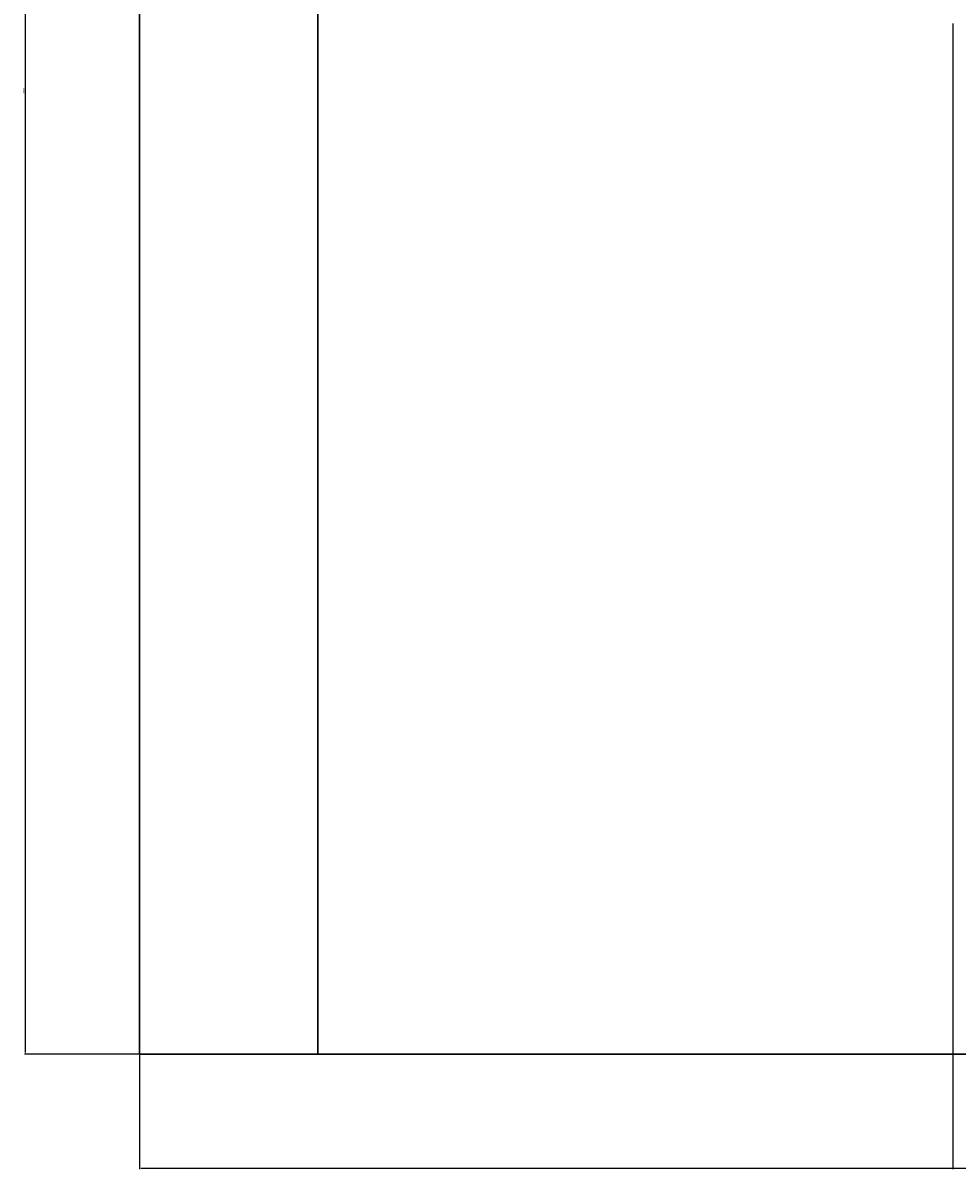
# Model space of a CAD drawing. Units: millimetres. Extents: x 2332 to 5836, y -853 to 2199.
# Tile 1 of 16: x 2332 to 3641, y -853 to 753. Entities that reach past the tile are written whole.
import ezdxf

# ---------------------------------------------------------------- set-up
doc = ezdxf.new("R2010")
doc.units = ezdxf.units.MM
doc.layers.add('A-ANNO-DIMS', color=2, linetype='Continuous', lineweight=18)
doc.layers.add('A-WALL', color=8, linetype='Continuous', lineweight=30)
doc.styles.get("Standard").update_dxf_attribs({"font": 'arial.ttf'})
doc.dimstyles.new('ISO-25', dxfattribs={"dimtxt": 2.5, "dimasz": 2.5, "dimexe": 1.25, "dimexo": 0.625, "dimtad": 1, "dimtxsty": 'Standard', "dimcen": 2.5, "dimadec": 0, "dimazin": 0, "dimtfac": 1, "dimtmove": 0, "dimatfit": 3, "dimfxl": 1, "dimarcsym": 0})

# ---------------------------------------------------------------- blocks, each defined once
blk = doc.blocks.new('*D15')
at = {"layer": 'A-ANNO-DIMS', "color": 0, "lineweight": -2, "transparency": 16777216}
for p, q in [((2495, -692.8), (2495, -853.1)), ((5675, -692.8), (5675, -853.1)), ((2497.5, -851.8), (5672.5, -851.8))]:
    blk.add_line(p, q, dxfattribs=at)
at = {"layer": 'A-ANNO-DIMS', "color": 0, "transparency": 16777216}
for points in [[(2497.5, -851.4), (2497.5, -852.3), (2495, -851.8)], [(5672.5, -851.4), (5672.5, -852.3), (5675, -851.8)]]:
    blk.add_solid(points, dxfattribs=at)
at = {"layer": 'Defpoints', "color": 0, "transparency": 16777216}
for p in [(2495, -692.2), (5675, -692.2), (5675, -851.8)]:
    blk.add_point(p, dxfattribs=at)
at = {"layer": 'A-ANNO-DIMS', "color": 0, "transparency": 16777216, "insert": (4085, -849.9), "char_height": 2.5, "attachment_point": 5}
blk.add_mtext('3180', dxfattribs=at)
blk = doc.blocks.new('*D16')
at = {"layer": 'A-ANNO-DIMS', "color": 0, "lineweight": -2, "transparency": 16777216}
for p, q in [((2494.4, 2007.8), (2334.1, 2007.8)), ((2335.4, -689.7), (2335.4, 2005.3)), ((2494.4, -692.2), (2334.1, -692.2))]:
    blk.add_line(p, q, dxfattribs=at)
at = {"layer": 'A-ANNO-DIMS', "color": 0, "transparency": 16777216}
for points in [[(2335, 2005.3), (2335.8, 2005.3), (2335.4, 2007.8)], [(2335, -689.7), (2335.8, -689.7), (2335.4, -692.2)]]:
    blk.add_solid(points, dxfattribs=at)
at = {"layer": 'Defpoints', "color": 0, "transparency": 16777216}
for p in [(2335.4, 2007.8), (2495, 2007.8), (2495, -692.2)]:
    blk.add_point(p, dxfattribs=at)
at = {"layer": 'A-ANNO-DIMS', "color": 0, "transparency": 16777216, "insert": (2333.5, 657.8), "char_height": 2.5, "attachment_point": 5, "rotation": 90}
blk.add_mtext('2700', dxfattribs=at)
blk = doc.blocks.new('*D22')
at = {"layer": 'A-ANNO-DIMS', "color": 0, "lineweight": -2, "transparency": 16777216}
for p, q in [((3635, 752.2), (3635, -853.1)), ((4785, 752.2), (4785, -853.1)), ((3637.5, -851.8), (4782.5, -851.8))]:
    blk.add_line(p, q, dxfattribs=at)
at = {"layer": 'A-ANNO-DIMS', "color": 0, "transparency": 16777216}
for points in [[(3637.5, -851.4), (3637.5, -852.3), (3635, -851.8)], [(4782.5, -851.4), (4782.5, -852.3), (4785, -851.8)]]:
    blk.add_solid(points, dxfattribs=at)
at = {"layer": 'Defpoints', "color": 0, "transparency": 16777216}
for p in [(3635, 752.8), (4785, 752.8), (4785, -851.8)]:
    blk.add_point(p, dxfattribs=at)
at = {"layer": 'A-ANNO-DIMS', "color": 0, "transparency": 16777216, "insert": (4210, -849.9), "char_height": 2.5, "attachment_point": 5}
blk.add_mtext('1150', dxfattribs=at)

msp = doc.modelspace()

# ---------------------------------------------------------------- linework, layer by layer
at = {"layer": 'A-WALL'}
for p, q in [((2495.04, -692.197), (2495.04, 2007.803)), ((2745.04, -692.197), (2745.04, 2007.803)), ((2745.04, -692.197), (2495.04, -692.197)), ((3345.04, -692.197), (2745.04, -692.197)), ((3655.04, -692.197), (3345.04, -692.197))]:
    msp.add_line(p, q, dxfattribs=at)

# ---------------------------------------------------------------- dimensions: what is measured, and where the dimension line sits
at = {"layer": 'A-ANNO-DIMS'}
dim = msp.add_linear_dim(base=(2335.39, 2007.803), p1=(2495.04, -692.197), p2=(2495.04, 2007.803), angle=90, dimstyle='ISO-25', override={"dimdec": 0, "dimlfac": 1, "dimrnd": 0, "dimzin": 0, "dimdsep": 46, "dimlunit": 2}, dxfattribs=at)
dim.commit()
dim.dimension.update_dxf_attribs({"geometry": '*D16', "text_midpoint": (2333.488, 657.803)})
for base, p1, p2, picture, middle in [((4785.04, -851.847), (3635.04, 752.803), (4785.04, 752.803), '*D22', (4210.04, -849.945)), ((5675.04, -851.847), (2495.04, -692.197), (5675.04, -692.197), '*D15', (4085.04, -849.944))]:
    dim = msp.add_linear_dim(base=base, p1=p1, p2=p2, dimstyle='ISO-25', override={"dimdec": 0, "dimlfac": 1, "dimrnd": 0, "dimzin": 0, "dimdsep": 46, "dimlunit": 2}, dxfattribs=at)
    dim.commit()
    dim.dimension.update_dxf_attribs({"geometry": picture, "text_midpoint": middle})

doc.saveas('drawing.dxf')
